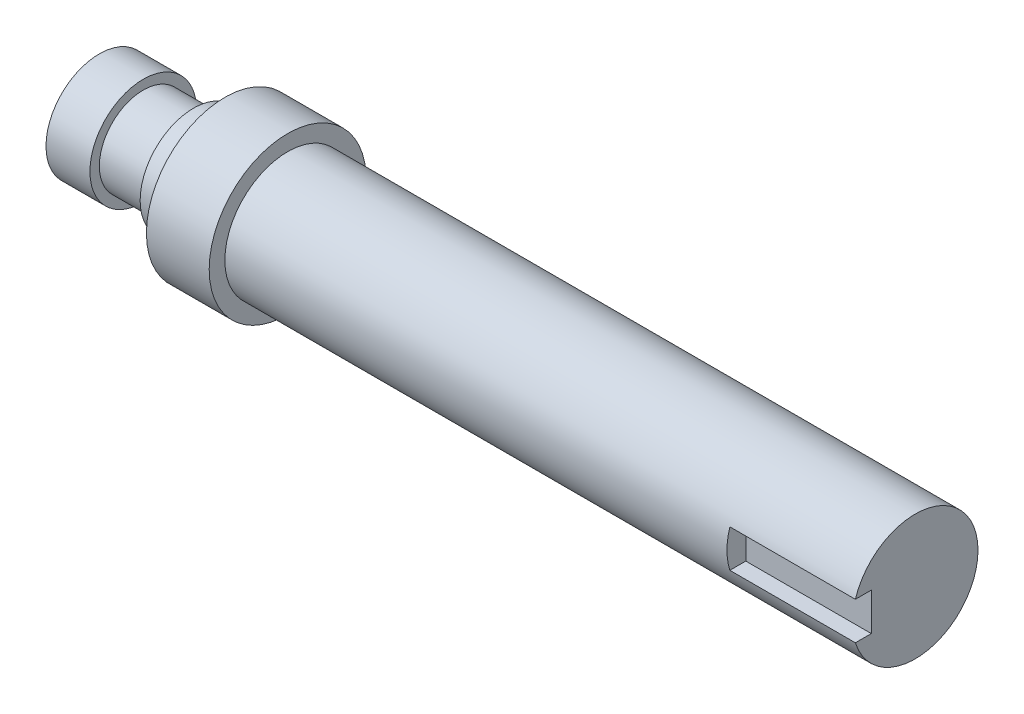
from build123d import *

# Parameters (mm, degrees)
KEYWAY_6X20_DEPTH_3_DEPTH = 3


with BuildPart() as part:
    # Shaft Profile Sketch → Stepped Shaft Body (revolve)
    with BuildSketch(Plane.XY, mode=Mode.PRIVATE) as stepped_shaft_body_sk:
        Polygon((0, 0), (130, 0), (130, -10), (30, -10), (30, -12.5), (20, -12.5), (20, -8.5), (15, -8.5), (15, -7), (7, -7), (7, -8.5), (0, -8.5), align=None)
    revolve(stepped_shaft_body_sk.sketch.rotate(Axis((0, 0, 0), (1, 0, 0)), 270), axis=Axis((0, 0, 0), (1, 0, 0)))

    # Keyway Sketch → Keyway 6x20 Depth 3 (cut)
    with BuildSketch(Plane.XY.offset(10)):
        Polygon((110, 0), (110, 3), (130, 3), (130, -3), (110, -3), align=None)
    extrude(amount=-KEYWAY_6X20_DEPTH_3_DEPTH, mode=Mode.SUBTRACT)


solid = part.part
